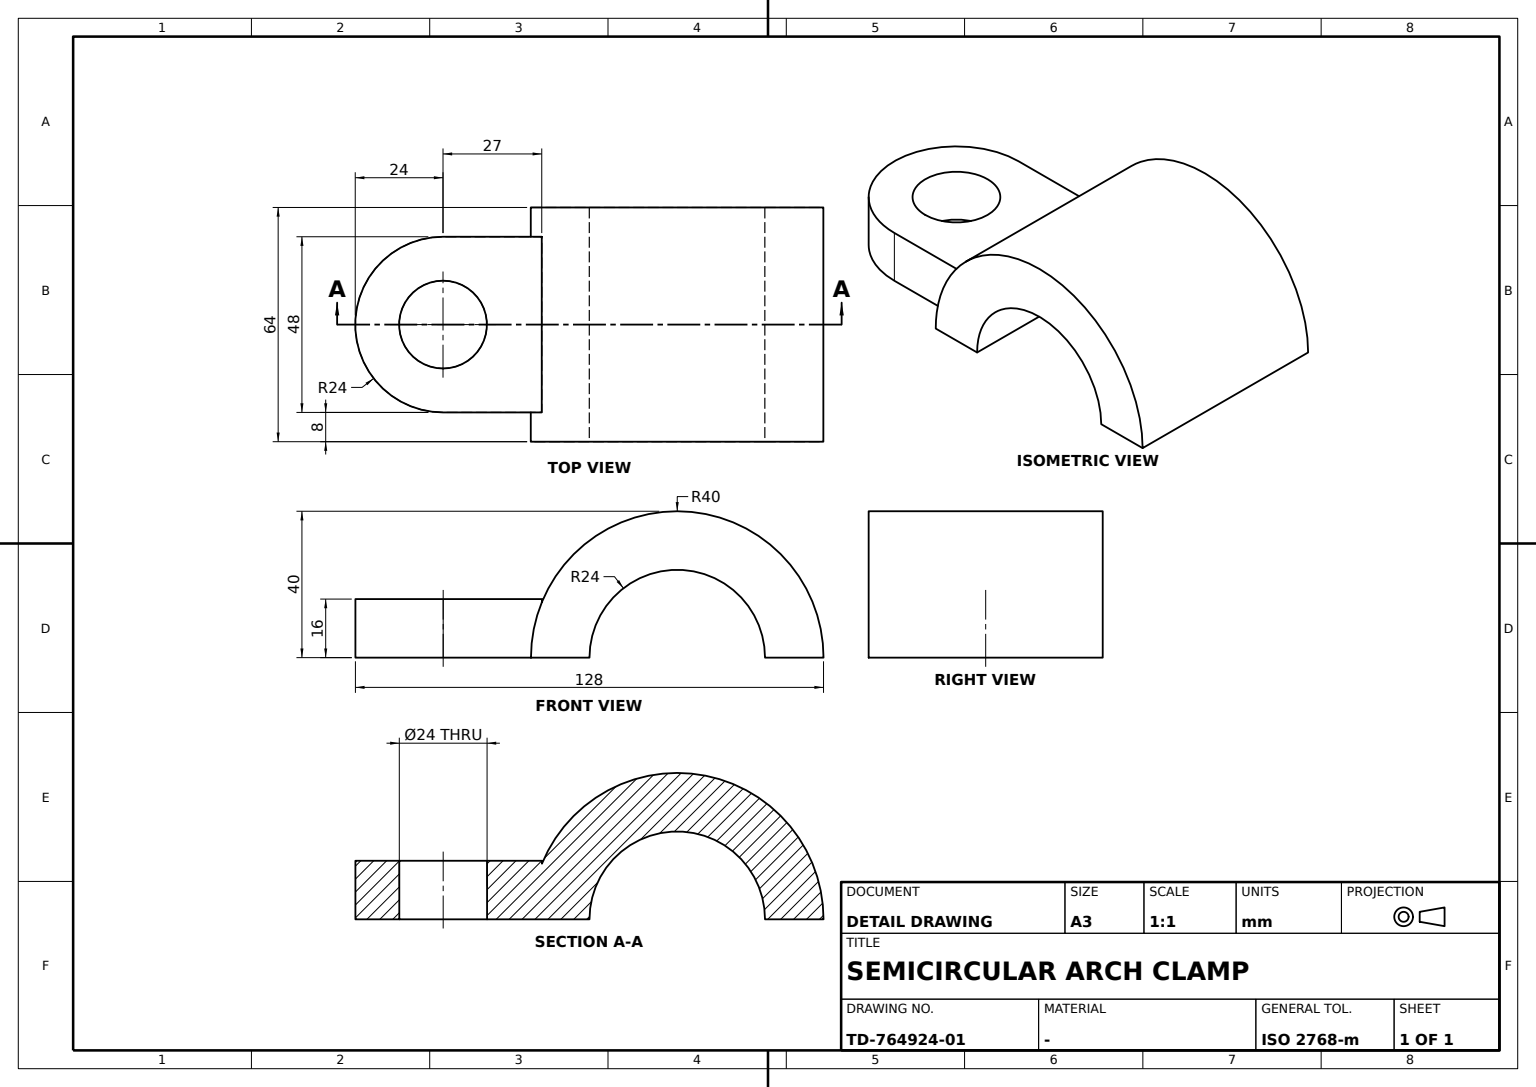
CATIA V5 part; units mm, degrees
sketch "Sketch1" plane through (0, 0, 0) normal (1, 0, 0) x (0, 1, 0)
  arc A0 (40, 0) -> (-40, 0) centre (0, 0) ccw
  arc A1 (24, 0) -> (-24, 0) centre (0, 0) ccw
  line L0 (-40, 0) -> (-24, 0)
  line L1 (24, 0) -> (40, 0)
  dimension "radius A0" = 40
  dimension "radius A1" = 24
  dimension "length L1" = 16
  constraint horizontal L0 x-axis
  constraint horizontal L1 x-axis
  constraint coincidence L0 L1
extrude "Pad1" add sketch "Sketch1" along normal mid plane 64
sketch "Sketch2" plane through (0, 0, 0) normal (0, 0, 1) x (1, 0, 0)
  line L0 (-24, -37) -> (24, -37)
  line L1 (24, -37) -> (24, -64)
  arc A0 (24, -64) -> (-24, -64) centre (0, -64) cw
  point P0 (0, -64)
  line L2 (-24, -64) -> (-24, -37)
  circle A1 centre (0, -64) radius 12
  dimension "radius A0" = 24
  dimension "radius A1" = 12
  dimension "distance x axis P0" = 64
  dimension "length L2" = 27
  dimension "distance L2 L1" = 48
  constraint horizontal L0 x-axis
  constraint vertical L1 y-axis
  constraint tangency A0 L1
  constraint symmetry L2 L1 y-axis
  constraint concentricity A0 A1
extrude "Pad2" add sketch "Sketch2" along normal blind 16
